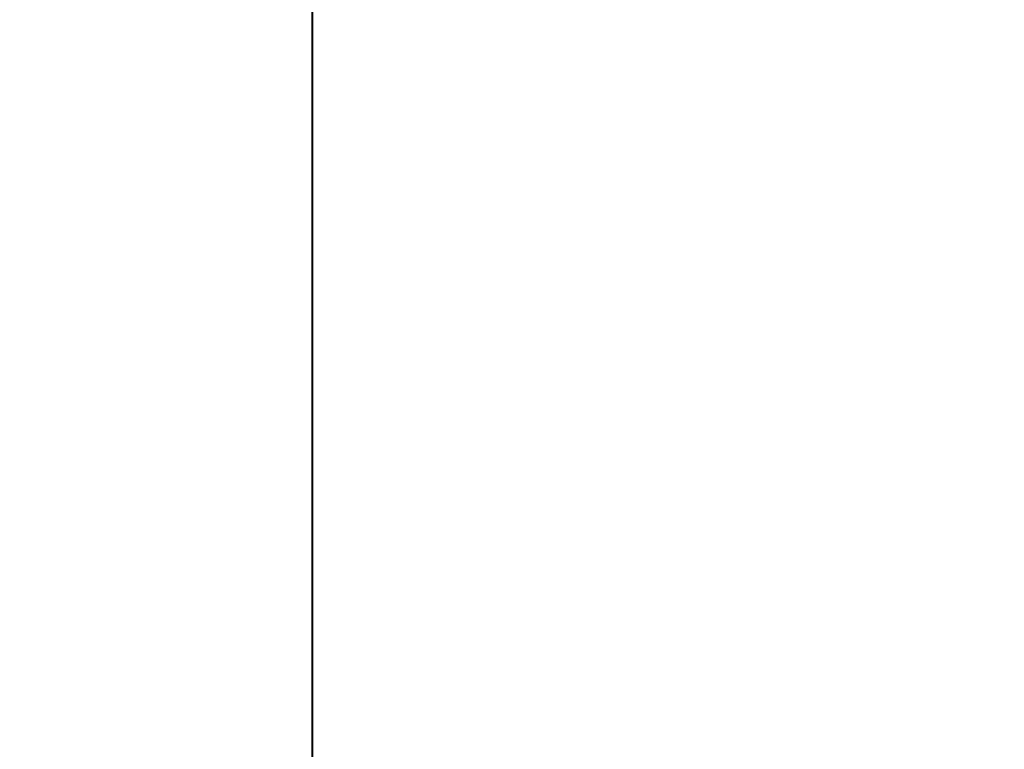
# Model space of a CAD drawing. Units: inches. Extents: x 459864 to 460310, y 324185 to 324787.
# Tile 88 of 112: x 460247.1043 to 460247.14006, y 324283.50868 to 324283.53519. Entities that reach past the tile are written whole.
import ezdxf

# ---------------------------------------------------------------- set-up
doc = ezdxf.new("R2010")
doc.units = ezdxf.units.IN
doc.layers.add('A-ANNO-DIMS', color=2, linetype='Continuous', lineweight=18)
doc.layers.add('A-WALL', color=7, linetype='Continuous', lineweight=40)
doc.styles.get("Standard").update_dxf_attribs({"font": 'arial.ttf'})
doc.dimstyles.new('ISO-25', dxfattribs={"dimtxt": 6, "dimasz": 2.5, "dimexe": 1.25, "dimexo": 0.625, "dimtad": 1, "dimdec": 1, "dimlunit": 3, "dimtxsty": 'Standard', "dimcen": 2.5, "dimadec": 0, "dimazin": 0, "dimtfac": 1, "dimtdec": 1, "dimtmove": 0, "dimatfit": 3, "dimfxl": 1, "dimarcsym": 0})

# ---------------------------------------------------------------- blocks, each defined once
blk = doc.blocks.new('*D21')
at = {"layer": 'A-ANNO-DIMS', "color": 0, "lineweight": -2, "transparency": 16777216}
for p, q in [((460247.739927, 324715.483233), (460309.580369, 324715.483233)), ((460308.330369, 324712.983233), (460308.330369, 324285.983233)), ((460247.739927, 324283.483233), (460309.580369, 324283.483233))]:
    blk.add_line(p, q, dxfattribs=at)
at = {"layer": 'A-ANNO-DIMS', "color": 0, "transparency": 16777216}
for points in [[(460307.913702, 324712.983233), (460308.747035, 324712.983233), (460308.330369, 324715.483233)], [(460307.913702, 324285.983233), (460308.747035, 324285.983233), (460308.330369, 324283.483233)]]:
    blk.add_solid(points, dxfattribs=at)
at = {"layer": 'Defpoints', "color": 0, "transparency": 16777216}
for p in [(460247.114927, 324715.483233), (460247.114927, 324283.483233), (460308.330369, 324283.483233)]:
    blk.add_point(p, dxfattribs=at)
at = {"layer": 'A-ANNO-DIMS', "color": 0, "transparency": 16777216, "insert": (460304.639884, 324499.483233), "char_height": 6, "attachment_point": 5, "rotation": 90}
blk.add_mtext("36'", dxfattribs=at)
blk = doc.blocks.new('*D62')
at = {"layer": 'A-ANNO-DIMS', "color": 0, "lineweight": -2, "transparency": 16777216}
for p, q in [((460247.739927, 324332.73872), (460278.764927, 324332.73872)), ((460277.514927, 324330.23872), (460277.514927, 324285.983233)), ((460247.739927, 324283.483233), (460278.764927, 324283.483233))]:
    blk.add_line(p, q, dxfattribs=at)
at = {"layer": 'A-ANNO-DIMS', "color": 0, "transparency": 16777216}
for points in [[(460277.09826, 324330.23872), (460277.931594, 324330.23872), (460277.514927, 324332.73872)], [(460277.09826, 324285.983233), (460277.931594, 324285.983233), (460277.514927, 324283.483233)]]:
    blk.add_solid(points, dxfattribs=at)
at = {"layer": 'Defpoints', "color": 0, "transparency": 16777216}
for p in [(460247.114927, 324332.73872), (460247.114927, 324283.483233), (460277.514927, 324283.483233)]:
    blk.add_point(p, dxfattribs=at)
at = {"layer": 'A-ANNO-DIMS', "color": 0, "transparency": 16777216, "insert": (460273.787608, 324308.110976), "char_height": 6, "attachment_point": 5, "rotation": 90}
blk.add_mtext('4\'-1 1/2"', dxfattribs=at)
blk = doc.blocks.new('*D67')
at = {"layer": 'A-ANNO-DIMS', "color": 0, "lineweight": -2, "transparency": 16777216}
for p, q in [((460208.114927, 324284.108233), (460208.114927, 324315.133233)), ((460247.114927, 324284.108233), (460247.114927, 324315.133233)), ((460210.614927, 324313.883233), (460244.614927, 324313.883233))]:
    blk.add_line(p, q, dxfattribs=at)
at = {"layer": 'A-ANNO-DIMS', "color": 0, "transparency": 16777216}
for points in [[(460210.614927, 324314.2999), (460210.614927, 324313.466566), (460208.114927, 324313.883233)], [(460244.614927, 324314.2999), (460244.614927, 324313.466566), (460247.114927, 324313.883233)]]:
    blk.add_solid(points, dxfattribs=at)
at = {"layer": 'Defpoints', "color": 0, "transparency": 16777216}
for p in [(460247.114927, 324313.883233), (460208.114927, 324283.483233), (460247.114927, 324283.483233)]:
    blk.add_point(p, dxfattribs=at)
at = {"layer": 'A-ANNO-DIMS', "color": 0, "transparency": 16777216, "insert": (460227.614927, 324317.573717), "char_height": 6, "attachment_point": 5}
blk.add_mtext('3\'-3"', dxfattribs=at)

msp = doc.modelspace()

# ---------------------------------------------------------------- linework, layer by layer
at = {"layer": 'A-WALL'}
msp.add_line((460247.114927, 324470.983233), (460247.114927, 324283.483233), dxfattribs=at)

# ---------------------------------------------------------------- dimensions: what is measured, and where the dimension line sits
at = {"layer": 'A-ANNO-DIMS'}
for base, p1, angle, override, picture, middle in [((460308.330369, 324283.483233), (460247.114927, 324715.483233), 90, {"dimclrd": 0, "dimclre": 0, "dimclrt": 0}, '*D21', (460304.639884, 324499.483233)), ((460277.514927, 324283.483233), (460247.114927, 324332.73872), 270, {"dimdec": 1, "dimlfac": 1, "dimrnd": 0, "dimzin": 1, "dimdsep": 46, "dimlunit": 4, "dimfrac": 2}, '*D62', (460273.787608, 324308.110976))]:
    dim = msp.add_linear_dim(base=base, p1=p1, p2=(460247.114927, 324283.483233), angle=angle, dimstyle='ISO-25', override=override, dxfattribs=at)
    dim.commit()
    dim.dimension.update_dxf_attribs({"geometry": picture, "text_midpoint": middle})
dim = msp.add_linear_dim(base=(460247.114927, 324313.883233), p1=(460208.114927, 324283.483233), p2=(460247.114927, 324283.483233), dimstyle='ISO-25', override={"dimdec": 1, "dimlfac": 1, "dimrnd": 0, "dimzin": 1, "dimdsep": 46, "dimlunit": 4, "dimfrac": 2}, dxfattribs=at)
dim.commit()
dim.dimension.update_dxf_attribs({"geometry": '*D67', "text_midpoint": (460227.614927, 324317.573717)})

doc.saveas('drawing.dxf')
